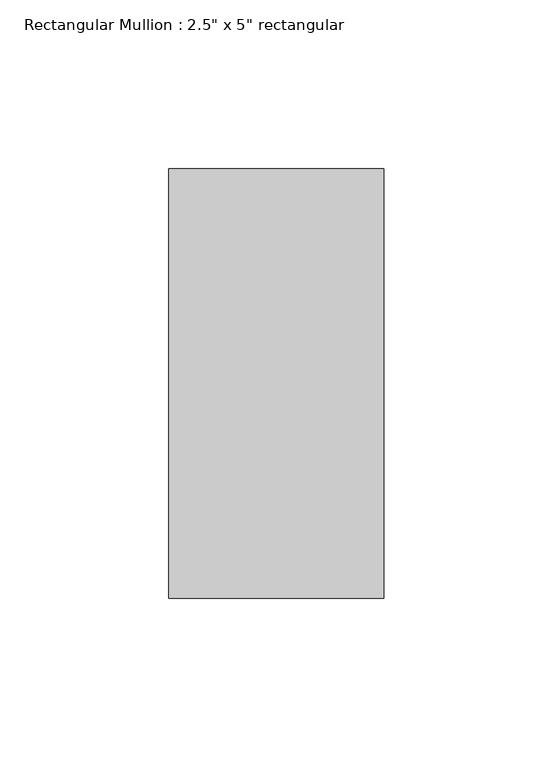
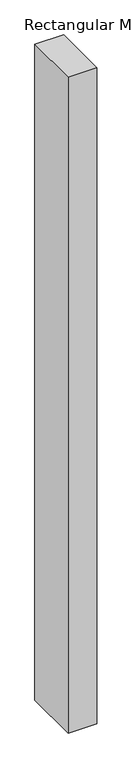
"""IFC4 building model written with IfcOpenShell, lengths in millimetres: member geometry."""

from ifc_helpers import new_model, si_unit, frame, origin, place, context, project, spatial, polyline, outline, extrude, source, transform, mapped, element, save


def member_1ff484d5(model_context):
    return source(origin(), model_context, "Body", "SweptSolid", [
        extrude(outline(polyline([(0.0, 63.5), (0.0, -63.5), (-63.5, -63.5), (-63.5, 63.5), (0.0, 63.5)])), frame((0.0, 0.0, -1529.3594037), z_axis=(0.0, 0.0, 1.0), x_axis=(1.0, 0.0, 0.0)), (0.0, 0.0, 1.0), 1529.3594037),
    ])


if __name__ == "__main__":
    model = new_model("IFC4")
    model_context = context("Model", 3, world=origin())
    ifc_project = project(units=[si_unit("LENGTHUNIT", "METRE", prefix="MILLI")], contexts=[model_context])
    site = spatial("IfcSite", under=ifc_project)
    building = spatial("IfcBuilding", under=site)
    placement = place(None, origin())
    member_shape = member_1ff484d5(model_context)
    element("IfcMember", 1, ObjectType="Rectangular Mullion : 2.5\" x 5\" rectangular", at=placement, inside=building, context=model_context, shape_type="MappedRepresentation", body=[
        mapped(member_shape, transform((0.0, 0.0, 0.0), x_axis=(1.0, 0.0, 0.0), y_axis=(0.0, 1.0, 0.0), z_axis=(0.0, 0.0, 1.0))),
    ])
    save(model, "model.ifc")

# Revit data of these elements
# Type "Rectangular Mullion : 2.5\" x 5\" rectangular"
#   built-in parameter 1007304 = 0.416667 (stored number, unit not read)
#   built-in parameter 1007301 = 0.104167 (stored number, unit not read)
#   built-in parameter 1007300 = 0.104167 (stored number, unit not read)
# Element 1 (IfcMember, "Rectangular Mullion : 2.5\" x 5\" rectangular")
#   Materials on its faces: "Aluminum"
# Materials
#   "Aluminum": class "Metal", colour RGB 247 247 247, transparency 0, Description = "Aluminum 6061", Cost = 0
